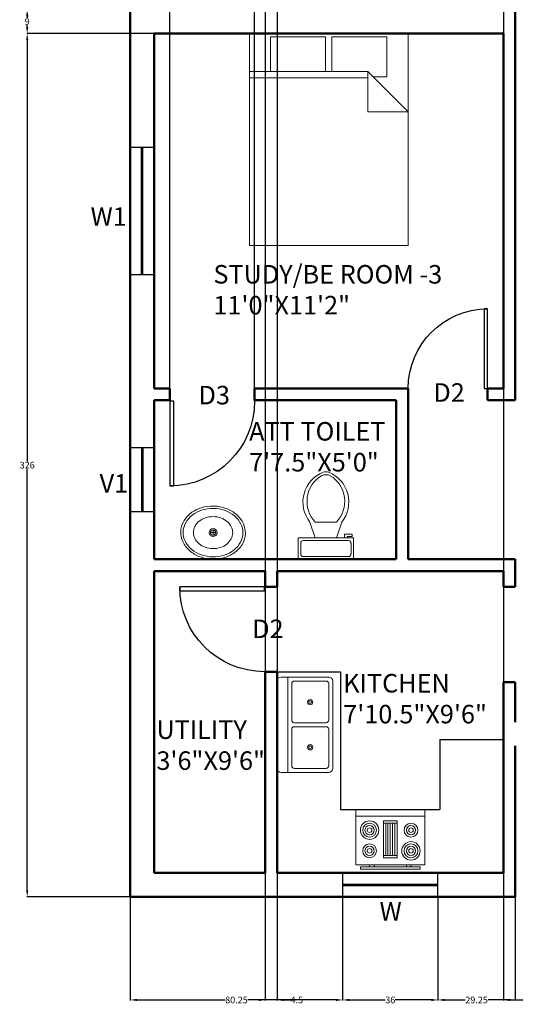
# Model space of a CAD drawing. Units: inches. Extents: x 227 to 711, y 218 to 1048.
# Tile 1 of 5: x 227 to 414, y 218 to 590. Entities that reach past the tile are written whole.
import ezdxf

# ---------------------------------------------------------------- set-up
doc = ezdxf.new("R2010")
doc.units = ezdxf.units.IN
doc.header["$MEASUREMENT"] = 0
for name, color, linetype, lineweight in [('A-ANNO-DIMS', 2, 'Continuous', 18), ('A-ANNO-TEXT', 70, 'Continuous', 18), ('A-AREA-IDEN', 70, 'Continuous', 25), ('A-FLOR-CASE', 32, 'Continuous', 25), ('A-FLOR-FIXT', 140, 'Continuous', 18), ('A-FURN', 8, 'Continuous', 18), ('A-WALL', 10, 'Continuous', 50), ('DOORS', 30, 'Continuous', 25), ('EQUIPMENTS', 140, 'Continuous', 18), ('WINDOWS', 50, 'Continuous', 25)]:
    doc.layers.add(name, color=color, linetype=linetype, lineweight=lineweight)
doc.styles.get("Standard").update_dxf_attribs({"font": 'arial.ttf'})
doc.dimstyles.get("Standard").update_dxf_attribs({"dimtxt": 2.5, "dimasz": 2.5, "dimexe": 0.18, "dimexo": 0.0625, "dimgap": 0.09, "dimtad": 0, "dimtih": 1, "dimtoh": 1, "dimzin": 0, "dimdsep": 46, "dimlunit": 3, "dimtxsty": 'Standard', "dimcen": 0.09, "dimadec": 0, "dimazin": 0, "dimtfac": 1, "dimtofl": 0, "dimtmove": 0, "dimatfit": 3, "dimfxl": 1, "dimtolj": 1, "dimtzin": 0, "dimarcsym": 0})

# ---------------------------------------------------------------- blocks, each defined once
blk = doc.blocks.new('*U2')
for p, q in [((0, 0), (0, -6)), ((40, 0), (40, -6))]:
    blk.add_line(p, q)
blk.add_lwpolyline([(0, 0), (0, 40), (1.75, 40), (1.75, 0)], close=True)
blk.add_arc((0, 0), 40, 0, 90)
blk = doc.blocks.new('Bed - Queen')
for p, q in [((0, -80.00003), (0, 0)), ((0, 0), (59.99999, 0)), ((59.99999, 0), (59.99999, -80.00003)), ((7.99999, -1.2), (28.79998, -1.2)), ((7.99999, -14.4), (7.99999, -1.2)), ((28.79998, -1.2), (28.79998, -14.4)), ((31.19999, -1.2), (51.99999, -1.2)), ((31.19999, -14.4), (31.19999, -1.2)), ((51.99999, -1.2), (51.99999, -16.4)), ((0, -14.4), (44.8, -14.4)), ((59.99999, -29.6), (44.8, -14.4)), ((44.8, -14.4), (44.8, -29.6)), ((44.8, -16.8), (0, -16.8)), ((51.99999, -16.4), (46.79936, -16.4)), ((44.8, -29.6), (59.99999, -29.6)), ((59.99999, -80.00003), (0, -80.00003))]:
    blk.add_line(p, q)
blk = doc.blocks.new('Toilet - top')
for p, q in [((9.5, -6), (9.5, -2)), ((-10, -8.5), (-8, -8.5)), ((-10, -9.5), (-10, -8.5)), ((-7, -9.5), (-10, -9.5)), ((-8, -8.5), (-8, -8)), ((-7, -8), (-7, -9.5)), ((-4, -8), (-6, -14)), ((4, -8), (6, -14)), ((4, -14), (-4, -14))]:
    blk.add_line(p, q)
blk.add_lwpolyline([(10.5, -8), (10.5, 0), (-10.5, 0), (-10.5, -8)], close=True)
for points in [[(-9.5, -2), (-9.5, -6)], [(8.5, -1), (-8.5, -1)], [(-8.5, -7), (8.5, -7)]]:
    blk.add_lwpolyline(points)
for centre, radius, start, end in [((-8.62, -1.88), 0.884, 81.8699, 188.1301), ((8.62, -1.88), 0.884, 351.8699, 98.1301), ((-8.62, -6.12), 0.884, 171.8699, 278.1301), ((8.62, -6.12), 0.884, 261.8699, 8.1301), ((3.52, -21.58), 12.17, 141.4691, 247.9714), ((4.2, -21.82), 11.33, 136.3677, 238.9468), ((-3.52, -21.58), 12.17, 292.0284, 38.5307), ((-4.2, -21.82), 11.33, 301.053, 43.6321), ((0, -27.88), 4, 245.7318, 294.2682), ((0, -29), 4, 254.8605, 285.1395)]:
    blk.add_arc(centre, radius, start, end)
blk = doc.blocks.new('Sink - Oval top')
for p, q in [((-1, 0), (1, 0)), ((0, 1), (0, -1))]:
    blk.add_line(p, q)
for points in [[(-12.23, 0.39, 0.117634), (-11.46, -3.36, 0.104469), (-8.88, -6.8, 0.090016), (-5.08, -9.07, 0.08192), (-0.32, -10.02, 0.08192), (4.49, -9.38, 0.090016), (8.42, -7.36, 0.104469), (11.22, -4.09, 0.117634), (12.23, -0.39, 0.117634), (11.46, 3.36, 0.104469), (8.88, 6.8, 0.090016), (5.08, 9.07, 0.08192), (0.32, 10.02, 0.08192), (-4.49, 9.38, 0.090016), (-8.42, 7.36, 0.104469), (-11.22, 4.09, 0.117634)], [(-11.29, 0.16, 0.118622), (-10.52, -3.25, 0.104678), (-8.07, -6.36, 0.089562), (-4.54, -8.37, 0.081185), (-0.13, -9.15, 0.081185), (4.3, -8.49, 0.089562), (7.89, -6.58, 0.104678), (10.42, -3.55, 0.118622), (11.29, -0.16, 0.118622), (10.52, 3.25, 0.104678), (8.07, 6.36, 0.089562), (4.54, 8.37, 0.081185), (0.13, 9.15, 0.081185), (-4.3, 8.49, 0.089562), (-7.89, 6.58, 0.104678), (-10.42, 3.55, 0.118622)], [(-7.42, 0.08, 0.118283), (-6.91, -2.17, 0.104607), (-5.29, -4.21, 0.089718), (-2.97, -5.53, 0.081436), (-0.07, -6.04, 0.081436), (2.84, -5.59, 0.089718), (5.2, -4.33, 0.104607), (6.86, -2.32, 0.118283), (7.42, -0.08, 0.118283), (6.91, 2.17, 0.104607), (5.29, 4.21, 0.089718), (2.97, 5.53, 0.081436), (0.07, 6.04, 0.081436), (-2.84, 5.59, 0.089718), (-5.2, 4.33, 0.104607), (-6.86, 2.32, 0.118283)]]:
    blk.add_lwpolyline(points, format="xyb", close=True)
for radius in [1.5, 1]:
    blk.add_circle((0, 0), radius)
blk = doc.blocks.new('Range-Oven - 30 in top')
for p, q in [((0, -3), (30, -3)), ((12, -6), (18, -6)), ((13, -20), (13, -6)), ((14, -6), (14, -20)), ((15, -20), (15, -6)), ((16, -6), (16, -20)), ((17, -20), (17, -6)), ((18, -20), (12, -20)), ((6, -24), (6, -25)), ((8, -25), (8, -24)), ((22, -25), (22, -24)), ((24, -24), (24, -25))]:
    blk.add_line(p, q)
for points in [[(0, -24), (0, 0), (30, 0), (30, -24)], [(12, -21), (12, -5), (18, -5), (18, -21)], [(2, -26), (2, -25), (28, -25), (28, -26)]]:
    blk.add_lwpolyline(points, close=True)
for centre, radius in [((6, -9), 4), ((6, -9), 3), ((6, -9), 2), ((6, -9), 1), ((24, -9), 3), ((24, -9), 2), ((24, -9), 1), ((6, -18), 3), ((6, -18), 2), ((6, -18), 1), ((24, -18), 4), ((24, -18), 3), ((24, -18), 2), ((24, -18), 1)]:
    blk.add_circle(centre, radius)
blk = doc.blocks.new('Sink-double - 36 in top')
for p, q in [((-18, -4), (18, -4)), ((-0.75, -18.5), (-0.75, -6.5)), ((0.75, -6.5), (0.75, -18.5))]:
    blk.add_line(p, q)
for points in [[(-16.5, 0), (16.5, 0)], [(-18, -19.5), (-18, -1.5)], [(18, -1.5), (18, -19.5)], [(-16.5, -18.5), (-16.5, -6.5)], [(-15.5, -5.5), (-1.75, -5.5)], [(1.75, -5.5), (15.5, -5.5)], [(16.5, -6.5), (16.5, -18.5)], [(16.5, -21), (-16.5, -21)], [(-1.75, -19.5), (-15.5, -19.5)], [(15.5, -19.5), (1.75, -19.5)]]:
    blk.add_lwpolyline(points)
for centre, radius in [((-8.5, -12.5), 1), ((-8.5, -12.5), 0.5), ((8.5, -12.5), 1), ((8.5, -12.5), 0.5)]:
    blk.add_circle(centre, radius)
for centre, radius, start, end in [((-16.5, -1.5), 1.5, 90, 180), ((16.5, -1.5), 1.5, 0, 90), ((-15.5, -6.5), 1, 90, 180), ((-1.75, -6.5), 1, 0, 90), ((1.75, -6.5), 1, 90, 180), ((15.5, -6.5), 1, 0, 90), ((-15.5, -18.5), 1, 180, 270), ((-1.75, -18.5), 1, 270, 0), ((1.75, -18.5), 1, 180, 270), ((15.5, -18.5), 1, 270, 0), ((-16.5, -19.5), 1.5, 180, 270), ((16.5, -19.5), 1.5, 270, 0)]:
    blk.add_arc(centre, radius, start, end)
blk = doc.blocks.new('WIN-48IN')
for p, q in [((0, 4.75), (48, 4.75)), ((0, 4.25), (48, 4.25))]:
    blk.add_line(p, q)
blk.add_lwpolyline([(0, 0), (48, 0), (48, 9), (0, 9)], close=True)
blk = doc.blocks.new('VENT-V1-24IN')
for p, q in [((4.25, 24), (4.25, 0)), ((4.75, 24), (4.75, 0))]:
    blk.add_line(p, q)
blk.add_lwpolyline([(0, 24), (0, 0), (9, 0), (9, 24)], close=True)
blk = doc.blocks.new('*D46')
at = {"layer": 'A-ANNO-DIMS', "color": 0, "lineweight": -2, "transparency": 16777216}
for p, q in [((268.99, 259), (268.99, 219.94)), ((349.24, 259), (349.24, 219.94)), ((271.49, 220.12), (304.8, 220.12)), ((346.74, 220.12), (313.43, 220.12))]:
    blk.add_line(p, q, dxfattribs=at)
at = {"layer": 'A-ANNO-DIMS', "color": 0, "transparency": 16777216}
for points in [[(271.49, 220.53), (271.49, 219.7), (268.99, 220.12)], [(346.74, 220.53), (346.74, 219.7), (349.24, 220.12)]]:
    blk.add_solid(points, dxfattribs=at)
at = {"layer": 'Defpoints', "color": 0, "transparency": 16777216}
for p in [(268.99, 259.07), (349.24, 259.07), (349.24, 220.12)]:
    blk.add_point(p, dxfattribs=at)
at = {"layer": 'A-ANNO-DIMS', "color": 0, "transparency": 16777216, "insert": (309.11, 220.12), "char_height": 2.5, "attachment_point": 5}
blk.add_mtext('\\A1;80.25', dxfattribs=at)
blk = doc.blocks.new('*D47')
at = {"layer": 'A-ANNO-DIMS', "color": 0, "lineweight": -2, "transparency": 16777216}
for p, q in [((349.24, 259), (349.24, 219.94)), ((385.24, 259), (385.24, 219.94)), ((351.74, 220.12), (365.36, 220.12)), ((382.74, 220.12), (369.12, 220.12))]:
    blk.add_line(p, q, dxfattribs=at)
at = {"layer": 'A-ANNO-DIMS', "color": 0, "transparency": 16777216}
for points in [[(351.74, 220.53), (351.74, 219.7), (349.24, 220.12)], [(382.74, 220.53), (382.74, 219.7), (385.24, 220.12)]]:
    blk.add_solid(points, dxfattribs=at)
at = {"layer": 'Defpoints', "color": 0, "transparency": 16777216}
for p in [(349.24, 259.07), (385.24, 259.07), (385.24, 220.12)]:
    blk.add_point(p, dxfattribs=at)
at = {"layer": 'A-ANNO-DIMS', "color": 0, "transparency": 16777216, "insert": (367.24, 220.12), "char_height": 2.5, "attachment_point": 5}
blk.add_mtext('\\A1;36', dxfattribs=at)
blk = doc.blocks.new('*D48')
at = {"layer": 'A-ANNO-DIMS', "color": 0, "lineweight": -2, "transparency": 16777216}
for p, q in [((385.24, 259), (385.24, 219.94)), ((414.49, 259), (414.49, 219.94)), ((387.74, 220.12), (395.53, 220.12)), ((411.99, 220.12), (404.2, 220.12))]:
    blk.add_line(p, q, dxfattribs=at)
at = {"layer": 'A-ANNO-DIMS', "color": 0, "transparency": 16777216}
for points in [[(387.74, 220.53), (387.74, 219.7), (385.24, 220.12)], [(411.99, 220.53), (411.99, 219.7), (414.49, 220.12)]]:
    blk.add_solid(points, dxfattribs=at)
at = {"layer": 'Defpoints', "color": 0, "transparency": 16777216}
for p in [(385.24, 259.07), (414.49, 259.07), (414.49, 220.12)]:
    blk.add_point(p, dxfattribs=at)
at = {"layer": 'A-ANNO-DIMS', "color": 0, "transparency": 16777216, "insert": (399.86, 220.12), "char_height": 2.5, "attachment_point": 5}
blk.add_mtext('\\A1;29.25', dxfattribs=at)
blk = doc.blocks.new('*D50')
at = {"layer": 'A-ANNO-DIMS', "color": 0, "lineweight": -2, "transparency": 16777216}
for p, q in [((277.93, 585.07), (229.86, 585.07)), ((230.04, 582.57), (230.04, 423.43)), ((230.04, 261.57), (230.04, 420.7)), ((268.93, 259.07), (229.86, 259.07))]:
    blk.add_line(p, q, dxfattribs=at)
at = {"layer": 'A-ANNO-DIMS', "color": 0, "transparency": 16777216}
for points in [[(229.62, 582.57), (230.46, 582.57), (230.04, 585.07)], [(229.62, 261.57), (230.46, 261.57), (230.04, 259.07)]]:
    blk.add_solid(points, dxfattribs=at)
at = {"layer": 'Defpoints', "color": 0, "transparency": 16777216}
for p in [(230.04, 585.07), (277.99, 585.07), (268.99, 259.07)]:
    blk.add_point(p, dxfattribs=at)
at = {"layer": 'A-ANNO-DIMS', "color": 0, "transparency": 16777216, "insert": (230.04, 422.07), "char_height": 2.5, "attachment_point": 5}
blk.add_mtext('\\A1;326', dxfattribs=at)
blk = doc.blocks.new('*D52')
at = {"layer": 'A-ANNO-DIMS', "color": 0, "lineweight": -2, "transparency": 16777216}
for p, q in [((277.93, 594.07), (229.86, 594.07)), ((230.04, 591.57), (230.04, 590.93)), ((230.04, 587.57), (230.04, 588.2)), ((277.93, 585.07), (229.86, 585.07))]:
    blk.add_line(p, q, dxfattribs=at)
at = {"layer": 'A-ANNO-DIMS', "color": 0, "transparency": 16777216}
for points in [[(229.62, 591.57), (230.46, 591.57), (230.04, 594.07)], [(229.62, 587.57), (230.46, 587.57), (230.04, 585.07)]]:
    blk.add_solid(points, dxfattribs=at)
at = {"layer": 'Defpoints', "color": 0, "transparency": 16777216}
for p in [(230.04, 594.07), (277.99, 594.07), (277.99, 585.07)]:
    blk.add_point(p, dxfattribs=at)
at = {"layer": 'A-ANNO-DIMS', "color": 0, "transparency": 16777216, "insert": (230.04, 589.57), "char_height": 2.5, "attachment_point": 5}
blk.add_mtext('\\A1;9', dxfattribs=at)
blk = doc.blocks.new('*D55')
at = {"layer": 'A-ANNO-DIMS', "color": 0, "lineweight": -2, "transparency": 16777216}
for p, q in [((283.99, 451.13), (283.99, 1046.2)), ((286.49, 1046.02), (298.12, 1046.02)), ((313.49, 1046.02), (301.86, 1046.02)), ((315.99, 451.13), (315.99, 1046.2))]:
    blk.add_line(p, q, dxfattribs=at)
at = {"layer": 'A-ANNO-DIMS', "color": 0, "transparency": 16777216}
for points in [[(286.49, 1046.43), (286.49, 1045.6), (283.99, 1046.02)], [(313.49, 1046.43), (313.49, 1045.6), (315.99, 1046.02)]]:
    blk.add_solid(points, dxfattribs=at)
at = {"layer": 'Defpoints', "color": 0, "transparency": 16777216}
for p in [(315.99, 1046.02), (283.99, 451.07), (315.99, 451.07)]:
    blk.add_point(p, dxfattribs=at)
at = {"layer": 'A-ANNO-DIMS', "color": 0, "transparency": 16777216, "insert": (299.99, 1046.02), "char_height": 2.5, "attachment_point": 5}
blk.add_mtext('\\A1;32', dxfattribs=at)
blk = doc.blocks.new('*D60')
at = {"layer": 'A-ANNO-DIMS', "color": 0, "lineweight": -2, "transparency": 16777216}
for p, q in [((459.49, 681), (459.49, 219.94)), ((409.99, 636), (409.99, 219.94)), ((412.49, 220.12), (431.34, 220.12)), ((456.99, 220.12), (438.14, 220.12))]:
    blk.add_line(p, q, dxfattribs=at)
at = {"layer": 'A-ANNO-DIMS', "color": 0, "transparency": 16777216}
for points in [[(412.49, 220.53), (412.49, 219.7), (409.99, 220.12)], [(456.99, 220.53), (456.99, 219.7), (459.49, 220.12)]]:
    blk.add_solid(points, dxfattribs=at)
at = {"layer": 'Defpoints', "color": 0, "transparency": 16777216}
for p in [(459.49, 681.07), (409.99, 636.07), (459.49, 220.12)]:
    blk.add_point(p, dxfattribs=at)
at = {"layer": 'A-ANNO-DIMS', "color": 0, "transparency": 16777216, "insert": (434.74, 220.12), "char_height": 2.5, "attachment_point": 5}
blk.add_mtext('\\A1;49.5', dxfattribs=at)
blk = doc.blocks.new('*D65')
at = {"layer": 'A-ANNO-DIMS', "color": 0, "lineweight": -2, "transparency": 16777216}
for p, q in [((319.99, 681), (319.99, 219.94)), ((324.49, 681), (324.49, 219.94)), ((317.49, 220.12), (314.99, 220.12)), ((326.99, 220.12), (329.49, 220.12))]:
    blk.add_line(p, q, dxfattribs=at)
at = {"layer": 'A-ANNO-DIMS', "color": 0, "transparency": 16777216}
for points in [[(317.49, 220.53), (317.49, 219.7), (319.99, 220.12)], [(326.99, 220.53), (326.99, 219.7), (324.49, 220.12)]]:
    blk.add_solid(points, dxfattribs=at)
at = {"layer": 'Defpoints', "color": 0, "transparency": 16777216}
for p in [(319.99, 681.07), (324.49, 681.07), (324.49, 220.12)]:
    blk.add_point(p, dxfattribs=at)
at = {"layer": 'A-ANNO-DIMS', "color": 0, "transparency": 16777216, "insert": (331.92, 220.12), "char_height": 2.5, "attachment_point": 5}
blk.add_mtext('\\A1;4.5', dxfattribs=at)

msp = doc.modelspace()

# ---------------------------------------------------------------- linework, layer by layer
at = {"layer": 'A-FLOR-CASE'}
for p, q in [((324.49, 344.065), (348.49, 344.065)), ((348.49, 344.065), (348.49, 292.065)), ((385.99, 318.436), (385.99, 292.065)), ((385.99, 318.436), (409.99, 318.436)), ((348.49, 292.065), (385.99, 292.065))]:
    msp.add_line(p, q, dxfattribs=at)
at = {"layer": 'A-WALL'}
for p, q in [((414.49, 594.065), (414.49, 446.565)), ((414.49, 594.065), (414.49, 585.065)), ((409.99, 585.065), (277.99, 585.065)), ((277.99, 585.065), (277.99, 451.065)), ((409.99, 585.065), (409.99, 451.065)), ((283.99, 451.065), (277.99, 451.065)), ((283.99, 451.065), (283.99, 446.565)), ((373.99, 451.065), (315.99, 451.065)), ((315.99, 451.065), (315.99, 446.565)), ((373.99, 451.065), (373.99, 386.565)), ((409.99, 451.065), (403.99, 451.065)), ((403.99, 451.065), (403.99, 446.565)), ((277.99, 446.565), (277.99, 386.565)), ((283.99, 446.565), (277.99, 446.565)), ((369.49, 446.565), (315.99, 446.565)), ((369.49, 446.565), (369.49, 386.565)), ((414.49, 446.565), (403.99, 446.565)), ((369.49, 386.565), (277.99, 386.565)), ((414.49, 386.565), (373.99, 386.565)), ((414.49, 386.565), (414.49, 376.065)), ((277.99, 382.065), (277.99, 268.065)), ((319.99, 382.065), (277.99, 382.065)), ((319.99, 382.065), (319.99, 376.065)), ((409.99, 382.065), (324.49, 382.065)), ((324.49, 382.065), (324.49, 376.065)), ((409.99, 382.065), (409.99, 376.065)), ((319.99, 376.065), (324.49, 376.065)), ((409.99, 376.065), (414.49, 376.065)), ((319.99, 344.065), (324.49, 344.065)), ((319.99, 344.065), (319.99, 268.065)), ((324.49, 344.065), (324.49, 268.065)), ((409.99, 340.065), (414.49, 340.065)), ((409.99, 340.065), (409.99, 268.065)), ((414.49, 340.065), (414.49, 325.065)), ((414.49, 316.065), (414.49, 259.065)), ((277.99, 268.065), (319.99, 268.065)), ((324.49, 268.065), (409.99, 268.065))]:
    msp.add_line(p, q, dxfattribs=at)
msp.add_lwpolyline([(414.49, 1007.065), (268.99, 1007.065), (268.99, 259.065), (414.49, 259.065)], dxfattribs=at)
at = {"layer": 'WINDOWS'}
for p, q in [((349.24, 263.815), (385.24, 263.815)), ((349.24, 263.315), (385.24, 263.315))]:
    msp.add_line(p, q, dxfattribs=at)
msp.add_lwpolyline([(349.24, 259.065), (385.24, 259.065), (385.24, 268.065), (349.24, 268.065)], close=True, dxfattribs=at)

# ---------------------------------------------------------------- block references
at = {"layer": 'A-FLOR-FIXT'}
for name, p, rotation in [('Toilet - top', (342.899, 386.565), 180), ('Sink-double - 36 in top', (324.49, 324.049), 90)]:
    msp.add_blockref(name, p, dxfattribs=dict(at, rotation=rotation))
msp.add_blockref('Sink - Oval top', (300.264, 396.589), dxfattribs=at)
at = {"layer": 'A-FURN'}
msp.add_blockref('Bed - Queen', (313.99, 585.065), dxfattribs=at)
at = {"layer": 'DOORS', "xscale": -0.7500000000000011, "yscale": 0.7500000000000011, "zscale": 0.7500000000000011}
msp.add_blockref('*U2', (403.99, 451.065), dxfattribs=at)
at = {"layer": 'DOORS', "xscale": -0.8, "yscale": 0.8, "zscale": 0.8}
for p, rotation in [((283.99, 446.265), 180), ((319.69, 376.065), 90)]:
    msp.add_blockref('*U2', p, dxfattribs=dict(at, rotation=rotation))
at = {"layer": 'EQUIPMENTS', "xscale": 0.8692268544197554, "yscale": 0.8692268544197554, "zscale": 0.8692268544197554}
msp.add_blockref('Range-Oven - 30 in top', (354.202, 292.065), dxfattribs=at)
at = {"layer": 'WINDOWS', "rotation": 90.00000000000006}
msp.add_blockref('WIN-48IN', (277.99, 494.065), dxfattribs=at)
at = {"layer": 'WINDOWS'}
msp.add_blockref('VENT-V1-24IN', (268.99, 404.565), dxfattribs=at)

# ---------------------------------------------------------------- texts
at = {"layer": 'A-ANNO-TEXT', "char_height": 7, "attachment_point": 1}
for s, insert in [('W1', (253.987, 519.442)), ('D3', (294.791, 452.005)), ('D2', (383.524, 453.003)), ('V1', (257.395, 418.678)), ('D2', (315.069, 363.764)), ('W', (363.183, 257.081))]:
    msp.add_mtext_dynamic_manual_height_columns(s, width=74.58955, gutter_width=1, heights=[0], dxfattribs=dict(at, insert=insert))
at = {"layer": 'A-AREA-IDEN', "char_height": 7, "attachment_point": 1}
for s, width, insert in [('STUDY/BE ROOM -3\\P11\'0"X11\'2"', 94.09069, (300.407, 497.639)), ('ATT TOILET\\P7\'7.5"X5\'0"', 74.58955, (313.911, 438.344)), ('KITCHEN\\P7\'10.5"X9\'6"', 74.58955, (349.466, 343.218)), ('UTILITY\\P3\'6"X9\'6"', 74.58955, (278.867, 325.666))]:
    msp.add_mtext_dynamic_manual_height_columns(s, width=width, gutter_width=1, heights=[0], dxfattribs=dict(at, insert=insert))

# ---------------------------------------------------------------- dimensions: what is measured, and where the dimension line sits
at = {"layer": 'A-ANNO-DIMS'}
for base, p1, p2, override, picture, middle in [((315.99, 1046.015), (283.99, 451.065), (315.99, 451.065), {"dimdec": 0, "dimlfac": 1, "dimrnd": 0, "dimzin": 0, "dimdsep": 46, "dimlunit": 2}, '*D55', (299.99, 1046.015)), ((324.49, 220.115), (319.99, 681.065), (324.49, 681.065), {"dimdec": 1, "dimlfac": 1, "dimrnd": 0, "dimzin": 0, "dimdsep": 46, "dimlunit": 2}, '*D65', (331.915, 220.115)), ((459.49, 220.115), (409.99, 636.065), (459.49, 681.065), {"dimdec": 1, "dimlfac": 1, "dimrnd": 0, "dimzin": 0, "dimdsep": 46, "dimlunit": 2}, '*D60', (434.74, 220.115)), ((349.24, 220.115), (268.99, 259.065), (349.24, 259.065), {"dimdec": 2, "dimlfac": 1, "dimrnd": 0, "dimzin": 0, "dimdsep": 46, "dimlunit": 2}, '*D46', (309.115, 220.115)), ((385.24, 220.115), (349.24, 259.065), (385.24, 259.065), {"dimdec": 0, "dimlfac": 1, "dimrnd": 0, "dimzin": 0, "dimdsep": 46, "dimlunit": 2}, '*D47', (367.24, 220.115)), ((414.49, 220.115), (385.24, 259.065), (414.49, 259.065), {"dimdec": 2, "dimlfac": 1, "dimrnd": 0, "dimzin": 0, "dimdsep": 46, "dimlunit": 2}, '*D48', (399.865, 220.115))]:
    dim = msp.add_linear_dim(base=base, p1=p1, p2=p2, dimstyle='Standard', override=override, dxfattribs=at)
    dim.commit()
    dim.dimension.update_dxf_attribs({"geometry": picture, "text_midpoint": middle})
for base, p1, p2, picture, middle in [((230.04, 594.065), (277.99, 585.065), (277.99, 594.065), '*D52', (230.04, 589.565)), ((230.04, 585.065), (268.99, 259.065), (277.99, 585.065), '*D50', (230.04, 422.065))]:
    dim = msp.add_linear_dim(base=base, p1=p1, p2=p2, angle=90, dimstyle='Standard', override={"dimdec": 0, "dimlfac": 1, "dimrnd": 0, "dimzin": 0, "dimdsep": 46, "dimlunit": 2}, dxfattribs=at)
    dim.commit()
    dim.dimension.update_dxf_attribs({"geometry": picture, "text_midpoint": middle})

doc.saveas('drawing.dxf')
